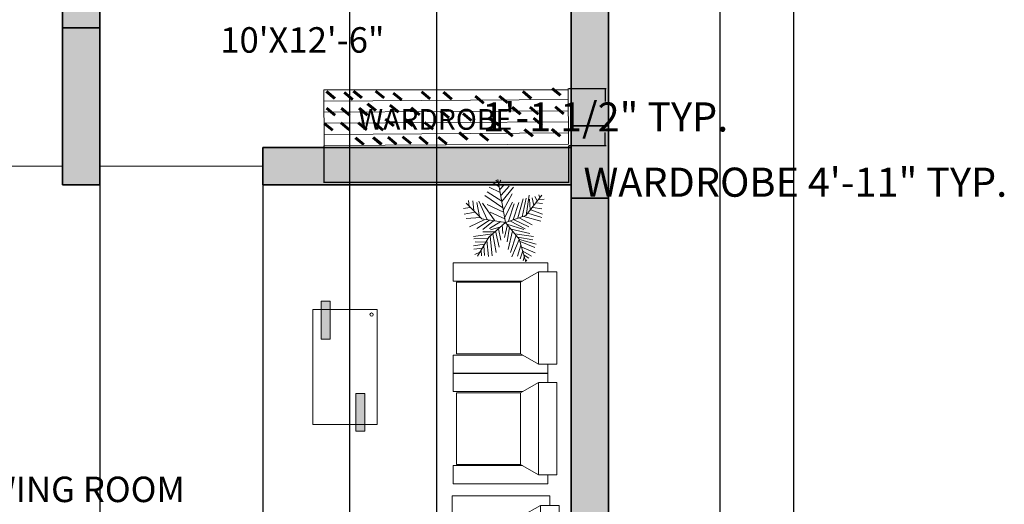
# Model space of a CAD drawing. Units: inches. Extents: x -17 to 892, y -721 to 172.
# Tile 9 of 11: x 655 to 892, y -231 to -115. Entities that reach past the tile are written whole.
import ezdxf

# ---------------------------------------------------------------- set-up
doc = ezdxf.new("R2010")
doc.units = ezdxf.units.IN
doc.header["$MEASUREMENT"] = 0
doc.layers.get('0').update_dxf_attribs({"color": 14})
for name, color, linetype, lineweight in [('A-ANNO-DIMS', 2, 'Continuous', 18), ('A-ANNO-TEXT', 7, 'Continuous', 18), ('A-AREA-IDEN', 7, 'Continuous', 18), ('A-COLS', 252, 'Continuous', 35), ('A-FLOR-CASE', 252, 'Continuous', 18), ('A-FURN-PATT', 252, 'Continuous', 9), ('A-WALL-PATT', 14, 'Continuous', 13), ('doors', 4, 'Continuous', 18), ('furniture', 252, 'Continuous', 18), ('lawn', 102, 'Continuous', 13), ('walls', 252, 'Continuous', 35)]:
    doc.layers.add(name, color=color, linetype=linetype, lineweight=lineweight)
doc.layers.add('A-COLS-PATT', color=254, linetype='Continuous', lineweight=13, true_color=0xd7ebd2)
doc.styles.get("Standard").update_dxf_attribs({"font": 'arial.ttf'})
doc.dimstyles.get("Standard").update_dxf_attribs({"dimtxt": 7, "dimasz": 0.18, "dimexe": 0.18, "dimexo": 0.0625, "dimgap": 0.09, "dimtad": 0, "dimtih": 1, "dimtoh": 1, "dimzin": 0, "dimdsep": 46, "dimlunit": 3, "dimtxsty": 'Standard', "dimcen": 0.09, "dimadec": 0, "dimazin": 0, "dimtfac": 1, "dimtofl": 0, "dimtmove": 0, "dimatfit": 3, "dimfxl": 1, "dimtolj": 1, "dimtzin": 0, "dimarcsym": 0})

# ---------------------------------------------------------------- blocks, each defined once
blk = doc.blocks.new('FABRIC SOFA 4S')
at = {"layer": 'furniture'}
for p, q in [((3, 54), (34, 54)), ((3, 51), (3, 54)), ((34, 48), (34, 54)), ((0, -51), (0, 51)), ((6, 51), (0, 51)), ((6, -51), (6, 51)), ((12, 47.63), (6, 51)), ((11.14, 48), (34, 48)), ((33, 23.81), (12, 23.81)), ((33, 0), (12, 0)), ((33, -23.81), (12, -23.81)), ((6, -51), (12, -47.63)), ((11.54, -48), (34, -48)), ((34, -48), (34, -54)), ((6, -51), (0, -51)), ((3, -54), (3, -51)), ((3, -54), (34, -54))]:
    blk.add_line(p, q, dxfattribs=at)
blk.add_lwpolyline([(12, -47.63), (12, 47.63), (33, 47.63), (33, -47.63)], close=True, dxfattribs=at)
blk = doc.blocks.new('FABRIC SOFA 1S')
at = {"layer": 'furniture'}
for p, q in [((3, 18.12), (34, 18.12)), ((3, 15.12), (3, 18.12)), ((34, 12.12), (34, 18.12)), ((0, -15.12), (0, 15.12)), ((6, 15.12), (0, 15.12)), ((6, -15.12), (6, 15.12)), ((12, 11.75), (6, 15.12)), ((11.33, 12.12), (34, 12.12)), ((6, -15.12), (12, -11.75)), ((11.33, -12.12), (34, -12.12)), ((34, -12.12), (34, -18.12)), ((6, -15.12), (0, -15.12)), ((3, -18.12), (3, -15.12)), ((3, -18.12), (34, -18.12))]:
    blk.add_line(p, q, dxfattribs=at)
blk.add_lwpolyline([(12, -11.75), (12, 11.75), (33, 11.75), (33, -11.75)], close=True, dxfattribs=at)
blk = doc.blocks.new('*U14')
for p, q in [((-8.737, 47.138), (-17.069, 52.711)), ((-10.186, 53.64), (-13.084, 55.962)), ((0, 0), (-10.5, 57)), ((-9.099, 51.782), (-6.563, 55.962)), ((-5.114, 28.097), (-24.676, 40.636)), ((-7.288, 39.707), (-21.778, 46.673)), ((-7.65, 43.423), (-2.578, 49.46)), ((-5.839, 35.992), (4.667, 48.067)), ((-5.114, 27.632), (10.463, 46.673)), ((-48.585, 21.131), (-49.309, 29.026)), ((-43.513, 28.561), (-42.427, 15.558)), ((-38.442, 26.239), (-34.819, 7.663)), ((-35.544, 28.097), (-24.314, 3.947)), ((-3.665, 19.273), (-27.574, 35.527)), ((-2.941, 16.486), (8.652, 37.85)), ((-1.129, 6.734), (9.014, 26.704)), ((10.101, 3.483), (17.708, 26.239)), ((16.259, 5.805), (23.142, 31.348)), ((22.055, 7.198), (27.489, 32.277)), ((27, 9), (48, 36)), ((27.127, 9.056), (31.112, 35.992)), ((31.836, 30.883), (32.561, 16.486)), ((35.096, 32.741), (37.27, 22.524)), ((38.719, 34.134), (41.979, 28.561)), ((43.791, 29.954), (51.036, 30.883)), ((44.153, 36.456), (45.239, 32.741)), ((-47.498, 19.737), (-55.83, 18.344)), ((-40.615, 13.7), (-55.105, 10.913)), ((-31.5, 4.5), (-52.5, 25.5)), ((-14.533, 2.09), (-30.834, 25.31)), ((-24.314, 23.917), (-2.941, 13.7)), ((-20.691, 13.7), (-1.129, 4.876)), ((3.942, 1.625), (11.187, 24.381)), ((33.285, 16.486), (48.862, 10.913)), ((36.183, 19.737), (48.137, 17.88)), ((40.53, 25.775), (48.862, 24.846)), ((-33.37, 6.269), (-52.207, 5.34)), ((-28.299, 3.483), (-47.86, -5.805)), ((-21.416, 3.018), (-38.079, -8.128)), ((0, 0), (-31.5, 4.5)), ((-15.982, 2.09), (-30.11, -9.521)), ((0, 0), (-22.5, -19.5)), ((-6.563, 1.161), (-21.416, -8.128)), ((0, 0), (27, 9)), ((0, 0), (18, -22.5)), ((6.478, 1.625), (26.04, -8.592)), ((11.187, 3.483), (30.749, -5.805)), ((18.07, 5.805), (35.096, -3.483)), ((24.229, 7.663), (46.688, 1.625)), ((29.662, 12.307), (48.137, 6.269)), ((-15.257, -12.772), (-30.11, -12.772)), ((-6.563, -5.805), (-19.967, -9.985)), ((-13.446, -11.378), (-8.737, -32.741)), ((-9.461, -8.592), (-6.201, -23.453)), ((-4.752, -3.483), (-3.665, -14.629)), ((2.493, -3.019), (-1.491, -20.202)), ((1.769, -2.555), (24.229, -9.521)), ((5.029, -6.27), (2.131, -25.775)), ((9.014, -11.378), (3.58, -35.992)), ((7.565, -9.056), (32.198, -14.629)), ((-17.431, -15.094), (-42.789, -18.809)), ((-24.314, -21.596), (-42.427, -22.06)), ((-26.849, -26.24), (-40.253, -25.775)), ((-22.5, -19.5), (-37.5, -45)), ((-25.038, -23.918), (-22.865, -45.281)), ((-20.691, -18.345), (-17.793, -44.352)), ((-17.069, -15.094), (-12.721, -40.172)), ((14.085, -16.951), (6.478, -40.172)), ((18.07, -22.524), (8.289, -45.745)), ((12.274, -15.094), (36.907, -18.809)), ((16.259, -19.738), (36.183, -22.989)), ((18, -22.5), (27, -52.5)), ((18.433, -22.524), (40.53, -29.026)), ((19.157, -25.311), (38.719, -33.206)), ((-28.299, -29.026), (-42.789, -31.348)), ((-30.834, -34.135), (-42.427, -35.528)), ((-32.646, -36.921), (-31.921, -44.352)), ((-29.023, -30.884), (-27.936, -43.887)), ((20.244, -30.419), (15.897, -44.816)), ((22.78, -37.85), (19.519, -48.532)), ((21.331, -32.741), (39.081, -40.636)), ((22.78, -38.314), (34.372, -44.816)), ((-34.457, -39.708), (-40.978, -42.494)), ((24.591, -45.745), (23.142, -50.854)), ((24.591, -43.423), (30.749, -47.603)), ((26.764, -49.925), (28.213, -50.854))]:
    blk.add_line(p, q)
blk = doc.blocks.new('*D17')
at = {"layer": 'A-ANNO-DIMS', "color": 0, "lineweight": -2, "transparency": 16777216}
for p, q in [((822.86, 89.9), (823.61, 89.9)), ((823.43, 89.72), (823.43, -263.08)), ((823.43, -623.21), (823.43, -270.41)), ((822.86, -623.39), (823.61, -623.39))]:
    blk.add_line(p, q, dxfattribs=at)
at = {"layer": 'A-ANNO-DIMS', "color": 0, "lineweight": 100, "transparency": 16777216}
for points in [[(823.4, 89.72), (823.46, 89.72), (823.43, 89.9)], [(823.4, -623.21), (823.46, -623.21), (823.43, -623.39)]]:
    blk.add_solid(points, dxfattribs=at)
at = {"layer": 'Defpoints', "color": 0, "lineweight": 100, "transparency": 16777216}
for p in [(822.8, 89.9), (822.8, -623.39), (823.43, -623.39)]:
    blk.add_point(p, dxfattribs=at)
at = {"layer": 'A-ANNO-DIMS', "color": 0, "transparency": 16777216, "insert": (823.43, -266.74), "char_height": 7, "attachment_point": 5}
blk.add_mtext('\\A1;57\'-1"', dxfattribs=at)
blk = doc.blocks.new('WARDROBE-59-PLAN')
for p, q in [((0, 13.37), (58.88, 13.37)), ((0.05, 13.37), (0.13, 0)), ((58.95, 0.34), (58.88, 13.71)), ((0.02, 10.69), (58.89, 11.04)), ((0.03, 8.02), (58.91, 8.36)), ((0.05, 5.35), (58.92, 5.69)), ((0.06, 2.67), (58.94, 3.02)), ((0.08, 0), (58.95, 0.34))]:
    blk.add_line(p, q)
blk = doc.blocks.new('TABLE-COCKTAIL')
h = blk.add_hatch(color=256)
h.dxf.hatch_style = 1
h.paths.add_polyline_path([(4.23, 29.31), (2.04, 29.31), (2.04, 22.19), (4.23, 22.19)])
h.paths.add_polyline_path([(4.23, 31.28), (2.04, 31.28), (2.04, 29.31), (4.23, 29.31)])
h.paths.add_polyline_path([(12.58, 9.09), (10.39, 9.09), (10.39, 1.62), (12.58, 1.62)])
h.paths.add_polyline_path([(12.58, 1.62), (10.39, 1.62), (10.39, 0), (12.58, 0)])
for p, q in [((2.04, 31.28), (4.23, 31.28)), ((2.04, 22.19), (2.04, 31.28)), ((4.23, 31.28), (4.23, 22.19)), ((0, 29.31), (0, 1.62)), ((15.53, 29.31), (0, 29.31)), ((15.53, 1.62), (15.53, 29.31)), ((4.23, 22.19), (2.04, 22.19)), ((10.39, 9.09), (12.58, 9.09)), ((10.39, 0), (10.39, 9.09)), ((12.58, 9.09), (12.58, 0)), ((0, 1.62), (15.53, 1.62)), ((12.58, 0), (10.39, 0))]:
    blk.add_line(p, q)
blk.add_circle((14.17, 28.1), 0.401)
blk = doc.blocks.new('*D40')
at = {"layer": 'A-ANNO-DIMS', "color": 0, "lineweight": -2, "transparency": 16777216}
for p, q in [((728.03, -144.94), (728.03, -153.9)), ((786.98, -144.94), (786.98, -153.9)), ((728.21, -153.72), (786.8, -153.72)), ((786.98, -153.72), (787.16, -153.72))]:
    blk.add_line(p, q, dxfattribs=at)
at = {"layer": 'A-ANNO-DIMS', "color": 0, "lineweight": 100, "transparency": 16777216}
for points in [[(728.21, -153.69), (728.21, -153.75), (728.03, -153.72)], [(786.8, -153.69), (786.8, -153.75), (786.98, -153.72)]]:
    blk.add_solid(points, dxfattribs=at)
at = {"layer": 'Defpoints', "color": 0, "lineweight": 100, "transparency": 16777216}
for p in [(728.03, -144.88), (786.98, -144.88), (786.98, -153.72)]:
    blk.add_point(p, dxfattribs=at)
at = {"layer": 'A-ANNO-DIMS', "color": 0, "transparency": 16777216, "insert": (841.6, -153.72), "char_height": 7, "attachment_point": 5}
blk.add_mtext('\\A1;WARDROBE 4\'-11" TYP.', dxfattribs=at)
blk = doc.blocks.new('*D41')
at = {"layer": 'A-ANNO-DIMS', "color": 0, "lineweight": -2, "transparency": 16777216}
for p, q in [((787.05, -131.17), (796.01, -131.17)), ((795.83, -131.35), (795.83, -134.31)), ((795.83, -144.7), (795.83, -141.73)), ((787.05, -144.88), (796.01, -144.88))]:
    blk.add_line(p, q, dxfattribs=at)
at = {"layer": 'A-ANNO-DIMS', "color": 0, "lineweight": 100, "transparency": 16777216}
for points in [[(795.8, -131.35), (795.86, -131.35), (795.83, -131.17)], [(795.8, -144.7), (795.86, -144.7), (795.83, -144.88)]]:
    blk.add_solid(points, dxfattribs=at)
at = {"layer": 'Defpoints', "color": 0, "lineweight": 100, "transparency": 16777216}
for p in [(786.98, -131.17), (795.83, -131.17), (786.98, -144.88)]:
    blk.add_point(p, dxfattribs=at)
at = {"layer": 'A-ANNO-DIMS', "color": 0, "transparency": 16777216, "insert": (795.83, -138.02), "char_height": 7, "attachment_point": 5}
blk.add_mtext('\\A1;1\'-1 1/2" TYP.', dxfattribs=at)
blk = doc.blocks.new('*D59')
at = {"layer": 'A-ANNO-DIMS', "color": 0, "lineweight": -2, "transparency": 16777216}
for p, q in [((796.64, 89.9), (841.36, 89.9)), ((841.18, 89.72), (841.18, -281.05)), ((841.18, -659.16), (841.18, -288.38)), ((796.64, -659.34), (841.36, -659.34))]:
    blk.add_line(p, q, dxfattribs=at)
at = {"layer": 'A-ANNO-DIMS', "color": 0, "lineweight": 100, "transparency": 16777216}
for points in [[(841.15, 89.72), (841.21, 89.72), (841.18, 89.9)], [(841.15, -659.16), (841.21, -659.16), (841.18, -659.34)]]:
    blk.add_solid(points, dxfattribs=at)
at = {"layer": 'Defpoints', "color": 0, "lineweight": 100, "transparency": 16777216}
for p in [(796.58, 89.9), (841.18, 89.9), (796.58, -659.34)]:
    blk.add_point(p, dxfattribs=at)
at = {"layer": 'A-ANNO-DIMS', "color": 0, "transparency": 16777216, "insert": (841.18, -284.72), "char_height": 7, "attachment_point": 5}
blk.add_mtext('\\A1;62\'-5"', dxfattribs=at)
blk = doc.blocks.new('*D62')
at = {"layer": 'A-ANNO-DIMS', "color": 0, "lineweight": -2, "transparency": 16777216}
for p, q in [((674.08, -154.45), (674.08, -704.12)), ((713.34, -154.45), (713.34, -704.12)), ((674.26, -703.94), (676.16, -703.94)), ((713.16, -703.94), (711.26, -703.94))]:
    blk.add_line(p, q, dxfattribs=at)
at = {"layer": 'A-ANNO-DIMS', "color": 0, "lineweight": 100, "transparency": 16777216}
for points in [[(674.26, -703.91), (674.26, -703.97), (674.08, -703.94)], [(713.16, -703.91), (713.16, -703.97), (713.34, -703.94)]]:
    blk.add_solid(points, dxfattribs=at)
at = {"layer": 'Defpoints', "color": 0, "lineweight": 100, "transparency": 16777216}
for p in [(674.08, -154.39), (713.34, -154.39), (713.34, -703.94)]:
    blk.add_point(p, dxfattribs=at)
at = {"layer": 'A-ANNO-DIMS', "color": 0, "transparency": 16777216, "insert": (693.71, -703.94), "char_height": 7, "attachment_point": 5}
blk.add_mtext('\\A1;3\'-3 1/2"', dxfattribs=at)
blk = doc.blocks.new('*D67')
at = {"layer": 'A-ANNO-DIMS', "color": 0, "lineweight": -2, "transparency": 16777216}
for p, q in [((734.21, 32.4), (734.21, -704.12)), ((755.21, 32.4), (755.21, -704.12)), ((734.39, -703.94), (735.64, -703.94)), ((755.03, -703.94), (753.77, -703.94))]:
    blk.add_line(p, q, dxfattribs=at)
at = {"layer": 'A-ANNO-DIMS', "color": 0, "lineweight": 100, "transparency": 16777216}
for points in [[(734.39, -703.91), (734.39, -703.97), (734.21, -703.94)], [(755.03, -703.91), (755.03, -703.97), (755.21, -703.94)]]:
    blk.add_solid(points, dxfattribs=at)
at = {"layer": 'Defpoints', "color": 0, "lineweight": 100, "transparency": 16777216}
for p in [(734.21, 32.46), (755.21, 32.46), (755.21, -703.94)]:
    blk.add_point(p, dxfattribs=at)
at = {"layer": 'A-ANNO-DIMS', "color": 0, "transparency": 16777216, "insert": (744.71, -703.94), "char_height": 7, "attachment_point": 5}
blk.add_mtext('\\A1;1\'-9"', dxfattribs=at)

msp = doc.modelspace()

# ---------------------------------------------------------------- hatches: boundary and pattern name
at = {"layer": 'A-COLS-PATT'}
h = msp.add_hatch(color=256, dxfattribs=at)
h.dxf.hatch_style = 1
h.paths.add_polyline_path([(796.576, 61.611), (787.576, 61.611), (787.576, 43.692), (796.576, 43.692)])
h.paths.add_polyline_path([(796.576, -140.181), (787.576, -140.181), (787.576, -157.529), (796.576, -157.529)])
h.paths.add_polyline_path([(674.076, -107.889), (665.076, -107.889), (665.076, -116.615), (674.076, -116.615)])
h.paths.add_polyline_path([(537.076, -107.889), (532.576, -107.889), (532.576, -116.615), (537.076, -116.615)])
h.paths.add_polyline_path([(541.576, -207.597), (532.576, -207.597), (532.576, -223.04), (541.576, -223.04)])
h.paths.add_polyline_path([(541.576, -335.389), (532.576, -335.389), (532.576, -350.421), (541.576, -350.421)])
h.paths.add_polyline_path([(541.576, -412.049), (532.576, -412.049), (532.576, -420.971), (541.576, -420.971)])
h.paths.add_polyline_path([(674.076, -410.999), (665.076, -410.999), (665.076, -421.003), (674.076, -421.003)])
h.paths.add_polyline_path([(674.076, -329.432), (665.076, -329.432), (665.076, -335.389), (665.076, -343.822), (674.076, -343.822), (674.076, -335.389)])
h.paths.add_polyline_path([(667.076, -610.134), (659.076, -610.134), (659.076, -618.889), (659.101, -623.389), (667.076, -623.389)])
h.paths.add_polyline_path([(796.576, -610.134), (787.576, -610.134), (787.576, -614.389), (787.576, -623.342), (796.576, -623.342)])
h.paths.add_polyline_path([(796.576, -324.682), (787.576, -324.682), (787.576, -353.487), (796.576, -353.487)])
at = {"layer": 'A-FURN-PATT'}
h = msp.add_hatch(dxfattribs=at)
h.set_pattern_fill('ANSI31', color=256, scale=0.84751258, angle=95.467005, style=0)
h.paths.add_polyline_path([(727.974, -139.792), (729.97, -141.44), (730.308, -141.031), (728.311, -139.383)])
h.paths.add_polyline_path([(735.524, -143.194), (737.52, -144.842), (737.858, -144.433), (735.861, -142.785)], flags=0)
h.paths.add_polyline_path([(732.034, -139.64), (734.031, -141.288), (734.368, -140.88), (732.372, -139.232)], flags=0)
h.paths.add_polyline_path([(728.545, -136.149), (730.542, -137.797), (730.88, -137.389), (728.883, -135.741)], flags=0)
h.paths.add_polyline_path([(739.789, -143.139), (741.786, -144.787), (742.123, -144.378), (740.126, -142.73)], flags=0)
h.paths.add_polyline_path([(736.179, -139.689), (738.176, -141.337), (738.513, -140.929), (736.516, -139.281)], flags=0)
h.paths.add_polyline_path([(732.12, -136.128), (734.117, -137.776), (734.454, -137.368), (732.457, -135.72)], flags=0)
h.paths.add_polyline_path([(728.547, -132.099), (730.544, -133.747), (730.882, -133.339), (728.885, -131.691)], flags=0)
h.paths.add_polyline_path([(743.348, -143.117), (745.345, -144.765), (745.683, -144.357), (743.686, -142.709)], flags=0)
h.paths.add_polyline_path([(740.107, -139.788), (742.103, -141.436), (742.441, -141.028), (740.444, -139.38)], flags=0)
h.paths.add_polyline_path([(736.414, -136.103), (738.411, -137.751), (738.748, -137.343), (736.751, -135.695)], flags=0)
h.paths.add_polyline_path([(732.791, -132.398), (734.788, -134.046), (735.125, -133.637), (733.128, -131.989)], flags=0)
h.paths.add_polyline_path([(746.858, -142.972), (748.854, -144.62), (749.192, -144.211), (747.195, -142.563)], flags=0)
h.paths.add_polyline_path([(742.713, -138.739), (744.71, -140.388), (745.047, -139.979), (743.05, -138.331)], flags=0)
h.paths.add_polyline_path([(738.408, -135.019), (740.405, -136.667), (740.742, -136.259), (738.745, -134.611)], flags=0)
h.paths.add_polyline_path([(735.046, -131.977), (737.042, -133.625), (737.38, -133.216), (735.383, -131.568)], flags=0)
h.paths.add_polyline_path([(750.915, -142.984), (752.912, -144.632), (753.249, -144.223), (751.252, -142.575)], flags=0)
h.paths.add_polyline_path([(747.293, -138.713), (749.29, -140.361), (749.627, -139.952), (747.63, -138.304)], flags=0)
h.paths.add_polyline_path([(743.828, -135.373), (745.825, -137.021), (746.162, -136.612), (744.165, -134.964)], flags=0)
h.paths.add_polyline_path([(740.375, -131.997), (742.372, -133.646), (742.709, -133.237), (740.712, -131.589)], flags=0)
h.paths.add_polyline_path([(755.489, -143.036), (757.486, -144.684), (757.823, -144.275), (755.826, -142.627)], flags=0)
h.paths.add_polyline_path([(752.158, -139.537), (754.155, -141.185), (754.492, -140.777), (752.495, -139.129)], flags=0)
h.paths.add_polyline_path([(748.95, -136.03), (750.947, -137.678), (751.284, -137.269), (749.287, -135.621)], flags=0)
h.paths.add_polyline_path([(744.597, -132.504), (746.594, -134.152), (746.931, -133.744), (744.934, -132.096)], flags=0)
h.paths.add_polyline_path([(760.479, -142.025), (762.476, -143.673), (762.813, -143.264), (760.816, -141.616)], flags=0)
h.paths.add_polyline_path([(755.993, -136.815), (757.99, -138.463), (758.327, -138.054), (756.33, -136.406)], flags=0)
h.paths.add_polyline_path([(751.43, -132.219), (753.427, -133.867), (753.764, -133.458), (751.767, -131.81)], flags=0)
h.paths.add_polyline_path([(765.507, -142.241), (767.504, -143.889), (767.841, -143.48), (765.844, -141.832)], flags=0)
h.paths.add_polyline_path([(761.433, -137.397), (763.429, -139.045), (763.767, -138.636), (761.77, -136.988)], flags=0)
h.paths.add_polyline_path([(756.662, -132.311), (758.659, -133.959), (758.996, -133.55), (756.999, -131.902)], flags=0)
h.paths.add_polyline_path([(771.308, -141.245), (773.304, -142.893), (773.642, -142.485), (771.645, -140.837)], flags=0)
h.paths.add_polyline_path([(767.946, -138.592), (769.943, -140.24), (770.28, -139.831), (768.284, -138.183)], flags=0)
h.paths.add_polyline_path([(764.36, -133.266), (766.357, -134.914), (766.694, -134.506), (764.698, -132.858)], flags=0)
h.paths.add_polyline_path([(770.111, -133.232), (772.107, -134.88), (772.445, -134.472), (770.448, -132.824)], flags=0)
h.paths.add_polyline_path([(778.401, -138.53), (780.398, -140.178), (780.735, -139.77), (778.738, -138.122)], flags=0)
h.paths.add_polyline_path([(773.263, -135.887), (775.26, -137.535), (775.597, -137.127), (773.6, -135.479)], flags=0)
h.paths.add_polyline_path([(776.221, -141.216), (778.218, -142.864), (778.555, -142.456), (776.559, -140.808)], flags=0)
h.paths.add_polyline_path([(782.808, -141.178), (784.805, -142.826), (785.142, -142.417), (783.145, -140.769)], flags=0)
h.paths.add_polyline_path([(783.613, -135.827), (785.61, -137.475), (785.947, -137.066), (783.95, -135.418)], flags=0)
h.paths.add_polyline_path([(777.549, -135.862), (779.546, -137.51), (779.883, -137.102), (777.886, -135.454)], flags=0)
h.paths.add_polyline_path([(782.85, -131.377), (784.847, -133.025), (785.184, -132.617), (783.187, -130.969)], flags=0)
h.paths.add_polyline_path([(775.853, -132.101), (777.849, -133.749), (778.187, -133.341), (776.19, -131.693)], flags=0)
at = {"layer": 'A-WALL-PATT'}
h = msp.add_hatch(color=256, dxfattribs=at)
h.dxf.hatch_style = 1
h.paths.add_polyline_path([(669.576, 4.611), (787.576, 4.611), (787.576, 9.111), (669.576, 9.111), (669.576, 53.097), (665.076, 53.097), (665.076, -107.889), (669.576, -107.889)])
h.paths.add_polyline_path([(674.076, -116.615), (665.076, -116.615), (665.076, -154.389), (674.076, -154.389)])
h.paths.add_polyline_path([(787.576, -145.389), (713.344, -145.389), (713.344, -154.389), (787.576, -154.389)])
h.paths.add_polyline_path([(632.137, -145.389), (622.476, -145.389), (622.476, -154.389), (632.137, -154.389)])
h.paths.add_polyline_path([(554.583, -145.389), (537.076, -145.389), (537.076, -154.389), (554.583, -154.389)])
h.paths.add_polyline_path([(537.076, -145.389), (532.576, -145.389), (532.576, -154.389), (537.076, -154.389)])
h.paths.add_polyline_path([(537.076, -116.615), (532.576, -116.615), (532.576, -145.389), (537.076, -145.389)])
h.paths.add_polyline_path([(796.576, 43.692), (787.576, 43.692), (787.576, -140.181), (796.576, -140.181)])
h.paths.add_polyline_path([(541.576, -223.04), (532.576, -223.04), (532.576, -282.182), (537.076, -282.182), (541.576, -282.182)])
h.paths.add_polyline_path([(796.576, -157.529), (787.576, -157.529), (787.576, -324.682), (796.576, -324.682)])
h.paths.add_polyline_path([(554.583, -335.389), (541.576, -335.389), (541.576, -344.389), (554.583, -344.389)])
h.paths.add_polyline_path([(635.731, -335.389), (622.476, -335.389), (622.476, -344.389), (635.731, -344.389)])
h.paths.add_polyline_path([(541.576, -350.421), (532.576, -350.421), (532.576, -412.049), (541.576, -412.049)])
h.paths.add_polyline_path([(674.076, -343.822), (665.076, -343.822), (665.076, -410.999), (674.076, -410.999)])
h.paths.add_polyline_path([(667.076, -421.003), (665.076, -421.003), (659.076, -421.002), (659.076, -610.134), (667.076, -610.134)])
h.paths.add_polyline_path([(796.576, -353.487), (787.576, -353.487), (787.576, -610.134), (796.576, -610.134)])
h.paths.add_polyline_path([(787.576, -335.389), (775.362, -335.389), (775.362, -344.389), (787.576, -344.389)])
h.paths.add_polyline_path([(707.469, -335.389), (703.501, -335.389), (703.501, -344.389), (707.469, -344.389)])
h.paths.add_polyline_path([(695.494, 61.611), (676.541, 61.611), (676.541, 57.111), (695.494, 57.111)])
h.paths.add_polyline_path([(729.183, 61.611), (724.076, 61.611), (711.12, 61.611), (711.12, 57.111), (729.183, 57.111)])
h.paths.add_polyline_path([(787.576, 61.611), (735.904, 61.611), (735.904, 57.111), (787.576, 57.111)])

# ---------------------------------------------------------------- linework, layer by layer
at = {"layer": 'A-COLS'}
for p, q in [((665.076, -116.615), (674.076, -116.615)), ((787.576, -140.181), (796.576, -140.181)), ((787.576, -157.529), (796.576, -157.529))]:
    msp.add_line(p, q, dxfattribs=at)
at = {"layer": 'doors'}
for p, q in [((632.137, -149.889), (665.076, -149.889)), ((674.076, -149.889), (713.344, -149.889))]:
    msp.add_line(p, q, dxfattribs=at)
at = {"layer": 'walls'}
for p, q in [((787.576, 61.611), (787.576, -614.389)), ((796.576, 61.611), (796.576, -623.389)), ((665.076, -154.389), (665.076, -107.889)), ((674.076, -154.389), (674.076, -107.889)), ((713.344, -145.389), (787.576, -145.389)), ((713.344, -154.389), (713.344, -145.389)), ((665.076, -154.389), (674.076, -154.389)), ((713.344, -154.389), (787.576, -154.389))]:
    msp.add_line(p, q, dxfattribs=at)

# ---------------------------------------------------------------- block references
at = {"layer": 'A-FLOR-CASE'}
msp.add_blockref('WARDROBE-59-PLAN', (728.03, -144.879), dxfattribs=at)
at = {"layer": 'furniture'}
for name, p, xscale, yscale, zscale, rotation in [('FABRIC SOFA 1S', (784.182, -186.408), 0.7339463821036302, 0.7339463821036302, 0.7339463821036302, 180), ('FABRIC SOFA 1S', (784.182, -213.014), 0.7339463821036302, 0.7339463821036302, 0.7339463821036302, 180.0000000000007), ('FABRIC SOFA 4S', (784.756, -270.167), 0.7583822975527559, 0.7583822975527559, 0.7583822975527559, 180)]:
    msp.add_blockref(name, p, dxfattribs=dict(at, xscale=xscale, yscale=yscale, zscale=zscale, rotation=rotation))
msp.add_blockref('TABLE-COCKTAIL', (725.369, -213.665), dxfattribs=at)
at = {"layer": 'lawn', "xscale": 0.1813548619598531, "yscale": 0.1813548619598531, "zscale": 0.1813548619598531}
msp.add_blockref('*U14', (771.83, -163.386), dxfattribs=at)

# ---------------------------------------------------------------- texts
at = {"layer": 'A-ANNO-TEXT'}
msp.add_text('WARDROBE', height=5, dxfattribs=at).set_placement((736.349, -141.104))
at = {"layer": 'A-AREA-IDEN'}
for s, p in [('10\'X12\'-6"', (703.094, -122.563)), ('DRAWING ROOM', (630.34, -230.702))]:
    msp.add_text(s, height=6.1361, dxfattribs=at).set_placement(p)

# ---------------------------------------------------------------- dimensions: what is measured, and where the dimension line sits
at = {"layer": 'A-ANNO-DIMS'}
dim = msp.add_linear_dim(base=(841.176, 89.902), p1=(796.576, -659.336), p2=(796.576, 89.902), angle=90, dimstyle='Standard', override={"dimdec": 1, "dimlfac": 1, "dimrnd": 0, "dimzin": 1, "dimdsep": 46, "dimlunit": 4, "dimfrac": 2}, dxfattribs=at)
dim.commit()
dim.dimension.update_dxf_attribs({"geometry": '*D59', "text_midpoint": (841.176, -284.717)})
for base, p1, p2, text, override, picture, middle in [((823.427, -623.389), (822.802, 89.902), (822.802, -623.389), '57\'-1"', {"dimclrd": 0, "dimclre": 0, "dimclrt": 0}, '*D17', (823.427, -266.744)), ((795.827, -131.169), (786.984, -144.88), (786.984, -131.169), '<> TYP.', {"dimdec": 1, "dimlfac": 1, "dimrnd": 0, "dimzin": 1, "dimdsep": 46, "dimlunit": 4, "dimfrac": 2}, '*D41', (795.827, -138.024))]:
    dim = msp.add_linear_dim(base=base, p1=p1, p2=p2, angle=90, text=text, dimstyle='Standard', override=override, dxfattribs=at)
    dim.commit()
    dim.dimension.update_dxf_attribs({"geometry": picture, "text_midpoint": middle})
for base, p1, p2, picture, middle in [((755.209, -703.936), (734.209, 32.461), (755.209, 32.461), '*D67', (744.709, -703.936)), ((713.344, -703.936), (674.076, -154.389), (713.344, -154.389), '*D62', (693.71, -703.936))]:
    dim = msp.add_linear_dim(base=base, p1=p1, p2=p2, dimstyle='Standard', override={"dimdec": 1, "dimlfac": 1, "dimrnd": 0, "dimzin": 1, "dimdsep": 46, "dimlunit": 4, "dimfrac": 2}, dxfattribs=at)
    dim.commit()
    dim.dimension.update_dxf_attribs({"geometry": picture, "text_midpoint": middle})
dim = msp.add_linear_dim(base=(786.984, -153.723), p1=(728.03, -144.88), p2=(786.984, -144.88), text='WARDROBE <> TYP.', dimstyle='Standard', override={"dimdec": 1, "dimlfac": 1, "dimrnd": 0, "dimzin": 1, "dimdsep": 46, "dimlunit": 4, "dimfrac": 2}, dxfattribs=at)
dim.commit()
dim.dimension.update_dxf_attribs({"geometry": '*D40', "text_midpoint": (841.604, -153.723)})

doc.saveas('drawing.dxf')
